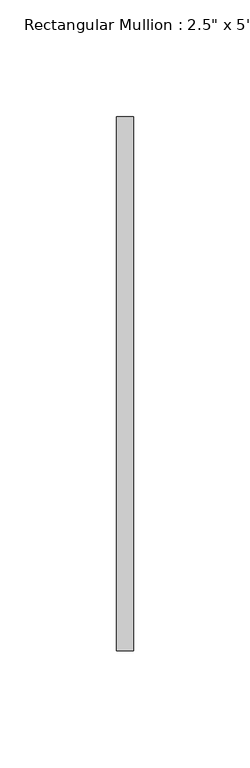
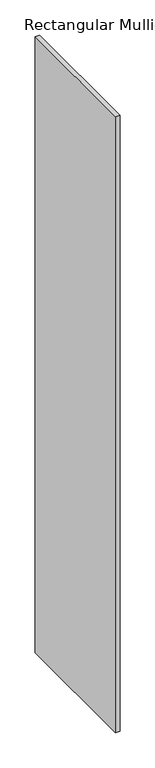
"""IFC4 building model written with IfcOpenShell, lengths in millimetres: member geometry."""

from ifc_helpers import new_model, si_unit, frame, origin, place, context, project, spatial, polyline, outline, extrude, source, transform, mapped, element, save


def member_05d02c6e(model_context):
    return source(origin(), model_context, "Body", "SweptSolid", [
        extrude(outline(polyline([(3.6195, 114.3), (3.6195, -114.3), (-3.6195, -114.3), (-3.6195, 114.3), (3.6195, 114.3)])), frame((0.0, 0.0, -1066.8), z_axis=(0.0, 0.0, 1.0), x_axis=(1.0, 0.0, 0.0)), (0.0, 0.0, 1.0), 1066.8),
    ])


if __name__ == "__main__":
    model = new_model("IFC4")
    model_context = context("Model", 3, world=origin())
    ifc_project = project(units=[si_unit("LENGTHUNIT", "METRE", prefix="MILLI")], contexts=[model_context])
    site = spatial("IfcSite", under=ifc_project)
    building = spatial("IfcBuilding", under=site)
    placement = place(None, origin())
    member_shape = member_05d02c6e(model_context)
    element("IfcMember", 1, ObjectType="Rectangular Mullion : 2.5\" x 5\" rectangular", at=placement, inside=building, context=model_context, shape_type="MappedRepresentation", body=[
        mapped(member_shape, transform((0.0, 0.0, 0.0), x_axis=(1.0, 0.0, 0.0), y_axis=(0.0, 1.0, 0.0), z_axis=(0.0, 0.0, 1.0))),
    ])
    save(model, "model.ifc")

# Revit data of these elements
# Type "Rectangular Mullion : 2.5\" x 5\" rectangular"
#   built-in parameter 1007304 = 0.75 (stored number, unit not read)
#   built-in parameter 1007301 = 0.011875 (stored number, unit not read)
#   built-in parameter 1007300 = 0.011875 (stored number, unit not read)
# Element 1 (IfcMember, "Rectangular Mullion : 2.5\" x 5\" rectangular")
#   Materials on its faces: "WINDOW GLASS MATERIAL"
# Materials
#   "WINDOW GLASS MATERIAL": class "Generic", colour RGB 120 120 120, transparency 0, Cost = 0
